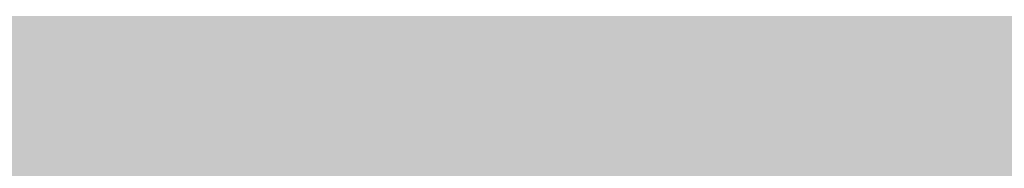
# Model space of a CAD drawing. Units: feet. Extents: x 3168 to 4724, y 827 to 1477.
# Tile 175 of 256: x 3303.032 to 3307.378, y 1098.344 to 1099.001. Entities that reach past the tile are written whole.
import ezdxf

# ---------------------------------------------------------------- set-up
doc = ezdxf.new("R2010")
doc.units = ezdxf.units.FT
doc.layers.add('A-ELEV', color=7, linetype='Continuous', lineweight=35)
doc.layers.add('A-ELEV-PATT', color=8, linetype='Continuous', lineweight=13)

msp = doc.modelspace()

# ---------------------------------------------------------------- hatches: boundary and pattern name
at = {"layer": 'A-ELEV-PATT'}
h = msp.add_hatch(color=256, dxfattribs=at)
h.dxf.hatch_style = 1
edge = h.paths.add_edge_path()
edge.add_ellipse((3552.9058, 979.2201), major_axis=(36.7449, 0), ratio=0.4848485, start_angle=0, end_angle=360)
edge = h.paths.add_edge_path()
edge.add_ellipse((3559.8916, 929.2523), major_axis=(36.7449, 0), ratio=0.4848485, start_angle=0, end_angle=360)
edge = h.paths.add_edge_path()
edge.add_line((3299.3168, 1198.6061), (3479.9167, 1198.6061))
edge.add_line((3479.9167, 1198.6061), (3479.9167, 1209.8686))
edge.add_spline(control_points=[(3479.9167, 1209.8686), (3464.3012, 1209.8686), (3448.6856, 1209.8686), (3410.9491, 1209.8686), (3388.8282, 1209.8686), (3355.6469, 1209.8686), (3344.5864, 1209.8686), (3327.9957, 1209.8686), (3322.4655, 1209.8686), (3314.1702, 1209.8686), (3311.4051, 1209.8686), (3307.2574, 1209.8686), (3305.8748, 1209.8686), (3303.801, 1209.8686), (3303.1097, 1209.8686), (3302.0728, 1209.8686), (3301.7272, 1209.8686), (3301.2087, 1209.8686), (3301.0359, 1209.8686), (3300.7767, 1209.8686), (3300.6903, 1209.8686), (3300.5606, 1209.8686), (3300.5174, 1209.8686), (3300.4526, 1209.8686), (3300.431, 1209.8686), (3300.3986, 1209.8686), (3300.3878, 1209.8686), (3300.3662, 1209.8686), (3300.3457, 1209.8686), (3300.3455, 1209.8686), (3300.3455, 1209.8686), (3300.3433, 1209.8686), (3300.3411, 1209.8686), (3300.3379, 1209.8686), (3300.3368, 1209.8686), (3300.3339, 1209.8686), (3300.3321, 1209.8686), (3300.3255, 1209.8686), (3300.3207, 1209.8686), (3300.3109, 1209.8686), (3300.306, 1209.8686), (3300.2905, 1209.8686), (3300.28, 1209.8686), (3300.2324, 1209.8688), (3300.1953, 1209.869), (3299.9511, 1209.8706), (3299.7448, 1209.8743), (3299.4368, 1209.8833), (3299.3344, 1209.8868), (3299.1811, 1209.8929), (3299.13, 1209.8951), (3298.6522, 1209.9168), (3298.2295, 1209.9457), (3297.6016, 1210.0024), (3297.3934, 1210.0235), (3297.0827, 1210.0583), (3296.9793, 1210.0705), (3296.293, 1210.1549), (3295.7181, 1210.2434), (3294.8687, 1210.3989), (3294.5877, 1210.4545), (3294.1693, 1210.5433), (3294.0304, 1210.5739), (3291.7071, 1211.1012), (3289.6536, 1211.8134), (3285.7763, 1213.564), (3283.9514, 1214.6035), (3280.5122, 1216.9801), (3278.8972, 1218.3176), (3276.3799, 1220.8295), (3275.416, 1221.9177), (3274.0393, 1223.7077), (3273.581, 1224.3495), (3273.1432, 1225.0163)], knot_values=[39.119033, 39.119033, 39.119033, 39.119033, 39.286353, 39.286353, 39.523379, 39.523379, 39.641892, 39.641892, 39.701148, 39.701148, 39.730777, 39.730777, 39.745591, 39.745591, 39.752998, 39.752998, 39.756701, 39.756701, 39.758553, 39.758553, 39.759479, 39.759479, 39.759942, 39.759942, 39.760173, 39.760173, 39.760289, 39.760289, 39.760405, 39.760405, 39.760463, 39.760463, 39.763389, 39.763389, 39.764851, 39.764851, 39.767304, 39.767304, 39.773825, 39.773825, 39.78057, 39.78057, 39.79477, 39.79477, 39.845194, 39.845194, 40.126715, 40.126715, 40.267476, 40.267476, 40.337856, 40.337856, 40.927023, 40.927023, 41.221606, 41.221606, 41.368898, 41.368898, 42.202622, 42.202622, 42.619485, 42.619485, 42.827916, 42.827916, 46.118323, 46.118323, 49.408731, 49.408731, 52.699139, 52.699139, 54.927489, 54.927489, 56.104228, 56.104228, 56.104228, 56.104228], weights=[1, 1, 1, 1, 1, 1, 1, 1, 1, 1, 1, 1, 1, 1, 1, 1, 1, 1, 1, 1, 1, 1, 1, 1, 1, 1, 1, 1, 1, 1, 1, 1, 1, 1, 1, 1, 1, 1, 1, 1, 1, 1, 1, 1, 1, 1, 1, 1, 1, 1, 1, 1, 1, 1, 1, 1, 1, 1, 1, 1, 1, 1, 1, 1, 1, 1, 1, 1, 1, 1, 1, 1, 1, 1], degree=3, periodic=0)
edge.add_line((3273.1432, 1225.0163), (3273.1432, 1099.0163))
edge.add_line((3273.1432, 1099.0163), (3299.3168, 1099.0163))
edge.add_line((3299.3168, 1099.0163), (3299.3168, 1198.6061))
edge = h.paths.add_edge_path()
edge.add_line((3304.7584, 1324.1581), (3479.9167, 1324.1581))
edge.add_line((3479.9167, 1324.1581), (3479.9167, 1335.7146))
edge.add_line((3479.9167, 1335.7146), (3269.1616, 1335.7146))
edge.add_spline(control_points=[(3269.1616, 1335.7146), (3264.0242, 1335.7146), (3258.3641, 1328.9582), (3259.2643, 1323.9003)], knot_values=[0, 0, 0, 0, 15.412191, 15.412191, 15.412191, 15.412191], degree=3, periodic=0)
edge.add_line((3259.2643, 1323.9003), (3265.5168, 1288.7691))
edge.add_line((3265.5168, 1288.7691), (3275.2651, 1261.5456))
edge.add_line((3275.2651, 1261.5456), (3304.7584, 1261.5456))
edge.add_line((3304.7584, 1261.5456), (3304.7584, 1324.1581))
h = msp.add_hatch(color=256, dxfattribs=at)
h.dxf.hatch_style = 1
h.paths.add_polyline_path([(3384.5252, 1099.0163), (3335.0292, 1099.0163), (3299.3168, 1099.0163), (3273.1432, 1099.0163), (3217.5654, 1099.0163), (3168.0693, 827.1163), (3335.0292, 827.1163)])

# ---------------------------------------------------------------- linework, layer by layer
at = {"layer": 'A-ELEV'}
msp.add_open_spline([(3808.5202, 1099.0163), (3808.5202, 1141.4132), (3808.5202, 1183.8102), (3808.5202, 1226.6353), (3808.5202, 1227.0636), (3808.5202, 1227.4918), (3811.4919, 1248.9947), (3814.4635, 1270.4975), (3817.4652, 1292.2176), (3817.4952, 1292.4348), (3817.5253, 1292.652), (3817.5728, 1310.1067), (3817.6203, 1327.5615), (3817.6679, 1345.0163), (3817.6679, 1345.458), (3817.6679, 1345.8996), (3817.6679, 1346.456), (3817.6679, 1346.5708), (3817.6679, 1346.7529), (3817.6679, 1346.8201), (3817.6679, 1346.9349), (3817.6679, 1346.9823), (3817.6679, 1347.0386), (3817.6679, 1347.0474), (3817.6679, 1347.0737), (3817.6679, 1347.0593), (3817.6679, 1347.0615), (3817.6679, 1347.0627), (3817.6679, 1347.066), (3817.6679, 1347.0683), (3817.6679, 1347.075), (3817.6679, 1347.0795), (3817.6678, 1347.0929), (3817.6678, 1347.1019), (3817.6678, 1347.1288), (3817.6677, 1347.1467), (3817.6674, 1347.2004), (3817.6672, 1347.2362), (3817.6661, 1347.3434), (3817.665, 1347.4147), (3817.6608, 1347.6281), (3817.6566, 1347.7697), (3817.64, 1348.1925), (3817.6235, 1348.4716), (3817.5591, 1349.3001), (3817.4961, 1349.8406), (3817.2554, 1351.4242), (3817.0263, 1352.4288), (3816.3069, 1354.8889), (3815.7437, 1356.2687), (3814.464, 1358.8192), (3813.7464, 1359.991), (3812.1958, 1362.1723), (3811.3622, 1363.1821), (3809.5888, 1365.069), (3808.6488, 1365.9461), (3806.6543, 1367.5796), (3805.5997, 1368.3362), (3803.3529, 1369.7223), (3802.1605, 1370.3524), (3799.6008, 1371.4536), (3798.2327, 1371.9255), (3795.2801, 1372.6346), (3793.6931, 1372.8721), (3791.8694, 1372.9265), (3791.7409, 1372.9292), (3791.3534, 1372.9341), (3791.0927, 1372.9329), (3790.3041, 1372.9151), (3789.7695, 1372.8842), (3789.2092, 1372.8302), (3789.1906, 1372.8284), (3789.1349, 1372.8229), (3789.0977, 1372.8191), (3789.0484, 1372.814), (3789.0364, 1372.8127), (3789.0003, 1372.8089), (3788.9761, 1372.8063), (3788.9494, 1372.8034), (3788.9468, 1372.8031), (3788.9426, 1372.8027), (3788.941, 1372.8025), (3788.9386, 1372.8022), (3788.9378, 1372.8021), (3788.9354, 1372.8019), (3788.8675, 1372.7944), (3788.7569, 1372.7822), (3788.7015, 1372.7761), (3788.5355, 1372.7579), (3788.4249, 1372.7457), (3788.0929, 1372.7092), (3787.8715, 1372.6848), (3787.2075, 1372.6118), (3786.7648, 1372.5631), (3785.4368, 1372.417), (3784.5515, 1372.3196), (3781.8954, 1372.0274), (3780.1247, 1371.8327), (3774.8126, 1371.2483), (3771.2713, 1370.8587), (3760.6471, 1369.69), (3753.5643, 1368.9109), (3732.316, 1366.5735), (3718.1504, 1365.0152), (3694.0068, 1362.3593), (3684.0287, 1361.2617), (3674.0506, 1360.1641), (3664.6007, 1360.1641), (3655.1508, 1360.1641), (3626.8011, 1360.1641), (3607.9013, 1360.1641), (3551.2019, 1360.1641), (3513.4023, 1360.1641), (3467.7252, 1360.1641), (3459.8476, 1360.1641), (3436.2149, 1360.1641), (3420.4597, 1360.1641), (3373.1943, 1360.1641), (3341.6839, 1360.1641), (3302.8482, 1360.1641), (3295.5227, 1360.1641), (3286.0383, 1360.1641), (3283.8794, 1360.1641), (3277.4026, 1360.1641), (3273.0848, 1360.1641), (3267.7329, 1360.1641), (3266.6988, 1360.1641), (3263.5965, 1360.1641), (3261.5284, 1360.1641), (3259.2369, 1360.1641), (3259.0137, 1360.1641), (3258.344, 1360.1641), (3257.8975, 1360.1641), (3257.431, 1360.1641), (3257.411, 1360.1641), (3257.3706, 1360.1641), (3257.3755, 1360.1641), (3257.3746, 1360.1641), (3257.3739, 1360.1641), (3257.372, 1360.1641), (3257.3706, 1360.1641), (3257.3667, 1360.1641), (3257.364, 1360.1641), (3257.3561, 1360.1641), (3257.3508, 1360.164), (3257.335, 1360.164), (3257.3244, 1360.164), (3257.2928, 1360.1639), (3257.2717, 1360.1638), (3257.2084, 1360.1634), (3257.1663, 1360.163), (3257.0402, 1360.1614), (3256.9563, 1360.1598), (3256.7055, 1360.1534), (3256.5392, 1360.147), (3256.0436, 1360.1219), (3255.7173, 1360.0971), (3254.7524, 1360.0005), (3254.128, 1359.9065), (3252.1801, 1359.5253), (3250.9416, 1359.144), (3248.6702, 1358.2433), (3247.6357, 1357.7238), (3245.7326, 1356.6035), (3244.8634, 1356.0021), (3243.2531, 1354.7429), (3242.512, 1354.0847), (3240.7511, 1352.3448), (3239.801, 1351.2296), (3238.0878, 1348.8724), (3237.3247, 1347.6304), (3235.9825, 1344.9716), (3235.4022, 1343.5549), (3234.5911, 1340.8155), (3234.3109, 1339.5435), (3233.9765, 1336.8026), (3233.9221, 1335.3309), (3234.1489, 1332.5913), (3234.3495, 1331.3672), (3234.7199, 1329.9994), (3234.7524, 1329.8834), (3234.8536, 1329.5348), (3234.9259, 1329.3017), (3235.0248, 1329.0026), (3235.0469, 1328.9369), (3235.0776, 1328.8472), (3235.0859, 1328.8232), (3235.1109, 1328.7511), (3235.1278, 1328.703), (3235.148, 1328.6462), (3235.1511, 1328.6376), (3235.1561, 1328.6235), (3235.1581, 1328.618), (3235.1602, 1328.612), (3235.1656, 1328.5969), (3235.1801, 1328.5565), (3235.1903, 1328.5281), (3235.2208, 1328.4429), (3235.2411, 1328.3862), (3235.3021, 1328.2159), (3235.3427, 1328.1023), (3235.4647, 1327.7617), (3235.546, 1327.5346), (3235.79, 1326.8534), (3235.9526, 1326.3992), (3236.4405, 1325.0367), (3236.7657, 1324.1284), (3237.7415, 1321.4034), (3238.392, 1319.5868), (3240.3435, 1314.1369), (3241.6445, 1310.5036), (3245.5476, 1299.6037), (3248.1496, 1292.3371), (3255.9557, 1270.5374), (3261.1598, 1256.0042), (3267.3876, 1238.612), (3268.4114, 1235.7529), (3269.5104, 1232.6839), (3269.5856, 1232.4739), (3269.7066, 1232.1359), (3269.7524, 1232.0079), (3269.8273, 1231.7987), (3269.8564, 1231.7176), (3269.9063, 1231.5781), (3269.9272, 1231.5198), (3269.9725, 1231.3934), (3269.9968, 1231.3254), (3270.0265, 1231.2425), (3270.0318, 1231.2277), (3270.0403, 1231.204), (3270.0392, 1231.207), (3270.0394, 1231.2066), (3270.0394, 1231.2064), (3270.0396, 1231.2058), (3270.0398, 1231.2055), (3270.0402, 1231.2043), (3270.0404, 1231.2036), (3270.0413, 1231.2013), (3270.0418, 1231.1998), (3270.0434, 1231.1953), (3270.0445, 1231.1922), (3270.0478, 1231.1832), (3270.0499, 1231.1771), (3270.0564, 1231.159), (3270.0608, 1231.147), (3270.0739, 1231.1108), (3270.0826, 1231.0867), (3270.1089, 1231.0144), (3270.1266, 1230.9663), (3270.1799, 1230.8225), (3270.2159, 1230.7269), (3270.3253, 1230.4415), (3270.4, 1230.2528), (3270.6292, 1229.6914), (3270.7889, 1229.3235), (3271.2865, 1228.2383), (3271.6431, 1227.5398), (3272.7759, 1225.5153), (3273.6142, 1224.2605), (3275.416, 1221.9177), (3276.3799, 1220.8295), (3278.8972, 1218.3176), (3280.5122, 1216.9801), (3283.9514, 1214.6035), (3285.7763, 1213.564), (3289.6536, 1211.8134), (3291.7071, 1211.1012), (3294.0304, 1210.5739), (3294.1693, 1210.5433), (3294.5877, 1210.4545), (3294.8687, 1210.3989), (3295.7181, 1210.2434), (3296.293, 1210.1549), (3296.9793, 1210.0705), (3297.0827, 1210.0583), (3297.3934, 1210.0235), (3297.6016, 1210.0024), (3298.2295, 1209.9457), (3298.6522, 1209.9168), (3299.13, 1209.8951), (3299.1811, 1209.8929), (3299.3344, 1209.8868), (3299.4368, 1209.8833), (3299.7448, 1209.8743), (3299.9511, 1209.8706), (3300.1953, 1209.869), (3300.2324, 1209.8688), (3300.28, 1209.8686), (3300.2905, 1209.8686), (3300.306, 1209.8686), (3300.3109, 1209.8686), (3300.3207, 1209.8686), (3300.3255, 1209.8686), (3300.3321, 1209.8686), (3300.3339, 1209.8686), (3300.3368, 1209.8686), (3300.3379, 1209.8686), (3300.3411, 1209.8686), (3300.3433, 1209.8686), (3300.3455, 1209.8686), (3300.3455, 1209.8686), (3300.3457, 1209.8686), (3300.3662, 1209.8686), (3300.3878, 1209.8686), (3300.3986, 1209.8686), (3300.431, 1209.8686), (3300.4526, 1209.8686), (3300.5174, 1209.8686), (3300.5606, 1209.8686), (3300.6903, 1209.8686), (3300.7767, 1209.8686), (3301.0359, 1209.8686), (3301.2087, 1209.8686), (3301.7272, 1209.8686), (3302.0728, 1209.8686), (3303.1097, 1209.8686), (3303.801, 1209.8686), (3305.8748, 1209.8686), (3307.2574, 1209.8686), (3311.4051, 1209.8686), (3314.1702, 1209.8686), (3322.4655, 1209.8686), (3327.9957, 1209.8686), (3344.5864, 1209.8686), (3355.6469, 1209.8686), (3388.8282, 1209.8686), (3410.9491, 1209.8686), (3477.3119, 1209.8686), (3521.5537, 1209.8686), (3566.8362, 1209.8686), (3567.8769, 1209.8686), (3570.999, 1209.8686), (3573.0804, 1209.8686), (3575.7814, 1209.8686), (3576.4009, 1209.8686), (3577.2958, 1209.8686), (3577.5712, 1209.8686), (3578.3971, 1209.8686), (3578.9478, 1209.8686), (3579.7565, 1209.8686), (3580.0145, 1209.8686), (3580.3427, 1209.8686), (3580.3269, 1209.8686), (3580.3272, 1209.8686), (3580.3273, 1209.8686), (3580.3278, 1209.8686), (3580.3281, 1209.8686), (3580.329, 1209.8686), (3580.3296, 1209.8686), (3580.3314, 1209.8686), (3580.3327, 1209.8686), (3580.3363, 1209.8686), (3580.3388, 1209.8686), (3580.3461, 1209.8686), (3580.351, 1209.8686), (3580.3657, 1209.8685), (3580.3754, 1209.8685), (3580.4048, 1209.8684), (3580.4244, 1209.8684), (3580.4832, 1209.8681), (3580.5224, 1209.8678), (3580.6404, 1209.8666), (3580.7192, 1209.8655), (3580.9563, 1209.8608), (3581.1152, 1209.8561), (3581.5942, 1209.8372), (3581.9164, 1209.8183), (3582.8899, 1209.7424), (3583.548, 1209.6662), (3585.5318, 1209.3606), (3586.8672, 1209.0539), (3589.4715, 1208.2525), (3590.7402, 1207.7579), (3591.9955, 1207.1588), (3592.0578, 1207.1287), (3592.2442, 1207.038), (3592.3677, 1206.9766), (3592.7353, 1206.7904), (3592.9768, 1206.6631), (3593.2445, 1206.5164), (3593.2747, 1206.4998), (3593.3651, 1206.4498), (3593.4251, 1206.4163), (3593.6043, 1206.3153), (3593.7227, 1206.2472), (3593.8572, 1206.1684), (3593.8744, 1206.1583), (3593.9257, 1206.128), (3593.9599, 1206.1078), (3594.0621, 1206.0469), (3594.1298, 1206.0061), (3594.2084, 1205.9582), (3594.2197, 1205.9513), (3594.2534, 1205.9307), (3594.2758, 1205.9169), (3594.343, 1205.8755), (3594.3876, 1205.8479), (3594.4336, 1205.819), (3594.4353, 1205.818), (3594.4402, 1205.8149), (3594.4435, 1205.8129), (3594.4471, 1205.8106), (3594.4475, 1205.8103), (3594.4487, 1205.8096), (3594.4495, 1205.8091), (3594.4504, 1205.8086), (3594.4505, 1205.8085), (3594.4506, 1205.8084), (3594.4674, 1205.7979), (3594.4933, 1205.7817), (3594.5062, 1205.7736), (3594.545, 1205.7492), (3594.5709, 1205.733), (3594.6485, 1205.6844), (3594.7002, 1205.652), (3594.8554, 1205.5547), (3594.9589, 1205.4898), (3595.2694, 1205.2953), (3595.4763, 1205.1656), (3596.0972, 1204.7765), (3596.5111, 1204.5171), (3597.7528, 1203.7388), (3598.5807, 1203.22), (3601.0642, 1201.6636), (3602.7198, 1200.6259), (3607.6868, 1197.513), (3610.9981, 1195.4377), (3620.932, 1189.2119), (3627.5546, 1185.0614), (3647.4225, 1172.6097), (3660.6678, 1164.3086), (3700.4035, 1139.4053), (3726.894, 1122.8031), (3757.2057, 1103.8061), (3761.027, 1101.4112), (3764.8482, 1099.0163), (3745.3283, 1099.0163), (3725.8083, 1099.0163), (3706.2884, 1099.0163), (3706.2884, 1108.4532), (3706.2884, 1117.8902), (3706.2884, 1127.3271), (3710.7508, 1127.3271), (3715.2131, 1127.3271), (3719.6755, 1127.3271)], degree=3, knots=[0, 0, 0, 0, 0.982037, 0.982037, 0.991957, 0.991957, 0.991957, 1.966522, 1.966522, 1.976367, 1.976367, 1.976367, 2.976367, 2.976367, 2.976367, 3.00169, 3.00169, 3.008272, 3.008272, 3.012129, 3.012129, 3.014851, 3.014851, 3.015353, 3.015353, 3.016359, 3.016359, 3.017365, 3.017365, 3.019376, 3.019376, 3.023398, 3.023398, 3.031442, 3.031442, 3.047531, 3.047531, 3.079708, 3.079708, 3.144063, 3.144063, 3.272772, 3.272772, 3.53019, 3.53019, 4.045026, 4.045026, 5.074698, 5.074698, 6.700878, 6.700878, 8.327058, 8.327058, 9.953238, 9.953238, 11.579418, 11.579418, 13.205598, 13.205598, 14.831778, 14.831778, 16.457958, 16.457958, 18.084138, 18.084138, 18.206872, 18.206872, 18.45234, 18.45234, 18.943275, 18.943275, 18.960093, 18.960093, 18.993729, 18.993729, 19.00461, 19.00461, 19.026374, 19.026374, 19.028737, 19.028737, 19.03018, 19.03018, 19.030897, 19.030897, 19.032332, 19.032332, 19.033766, 19.033766, 19.036636, 19.036636, 19.042374, 19.042374, 19.053851, 19.053851, 19.076805, 19.076805, 19.122714, 19.122714, 19.21453, 19.21453, 19.398163, 19.398163, 19.765429, 19.765429, 20.024128, 20.024128, 20.024128, 20.092031, 20.092031, 20.227836, 20.227836, 20.499446, 20.499446, 20.556051, 20.556051, 20.66926, 20.66926, 20.895678, 20.895678, 20.948316, 20.948316, 20.963829, 20.963829, 20.994855, 20.994855, 21.002285, 21.002285, 21.017146, 21.017146, 21.01875, 21.01875, 21.021959, 21.021959, 21.022102, 21.022102, 21.022249, 21.022249, 21.022708, 21.022708, 21.023627, 21.023627, 21.025464, 21.025464, 21.029138, 21.029138, 21.036486, 21.036486, 21.051183, 21.051183, 21.080575, 21.080575, 21.139361, 21.139361, 21.256932, 21.256932, 21.492073, 21.492073, 21.962356, 21.962356, 23.01002, 23.01002, 24.057684, 24.057684, 25.105348, 25.105348, 26.153011, 26.153011, 27.776787, 27.776787, 29.400562, 29.400562, 31.024337, 31.024337, 32.278801, 32.278801, 33.533265, 33.533265, 34.467568, 34.467568, 34.553971, 34.553971, 34.726776, 34.726776, 34.775309, 34.775309, 34.793079, 34.793079, 34.82862, 34.82862, 34.834979, 34.834979, 34.839039, 34.839039, 34.839411, 34.839411, 34.840285, 34.840285, 34.842034, 34.842034, 34.845531, 34.845531, 34.852525, 34.852525, 34.866512, 34.866512, 34.894488, 34.894488, 34.950439, 34.950439, 35.062342, 35.062342, 35.286147, 35.286147, 35.733758, 35.733758, 35.821815, 35.821815, 35.828283, 35.828283, 35.832225, 35.832225, 35.834724, 35.834724, 35.836521, 35.836521, 35.838617, 35.838617, 35.839073, 35.839073, 35.839345, 35.839345, 35.839617, 35.839617, 35.840161, 35.840161, 35.841249, 35.841249, 35.843425, 35.843425, 35.847778, 35.847778, 35.856482, 35.856482, 35.873891, 35.873891, 35.908709, 35.908709, 35.978345, 35.978345, 36.117617, 36.117617, 36.396161, 36.396161, 36.953248, 36.953248, 38.067423, 38.067423, 40.295772, 40.295772, 42.524122, 42.524122, 45.81453, 45.81453, 49.104937, 49.104937, 52.395345, 52.395345, 52.603776, 52.603776, 53.020639, 53.020639, 53.854363, 53.854363, 54.001655, 54.001655, 54.296238, 54.296238, 54.885405, 54.885405, 54.955785, 54.955785, 55.096546, 55.096546, 55.378067, 55.378067, 55.42849, 55.42849, 55.442691, 55.442691, 55.449436, 55.449436, 55.455957, 55.455957, 55.458409, 55.458409, 55.459872, 55.459872, 55.462798, 55.462798, 55.462856, 55.462856, 55.462972, 55.462972, 55.463088, 55.463088, 55.463319, 55.463319, 55.463782, 55.463782, 55.464708, 55.464708, 55.46656, 55.46656, 55.470263, 55.470263, 55.47767, 55.47767, 55.492484, 55.492484, 55.522112, 55.522112, 55.581369, 55.581369, 55.699882, 55.699882, 55.936907, 55.936907, 56.410959, 56.410959, 56.42211, 56.42211, 56.444413, 56.444413, 56.451051, 56.451051, 56.454001, 56.454001, 56.459901, 56.459901, 56.462666, 56.462666, 56.463418, 56.463418, 56.464171, 56.464171, 56.465675, 56.465675, 56.468684, 56.468684, 56.474702, 56.474702, 56.486738, 56.486738, 56.51081, 56.51081, 56.558955, 56.558955, 56.655243, 56.655243, 56.847821, 56.847821, 57.232975, 57.232975, 58.003284, 58.003284, 59.543901, 59.543901, 62.625137, 62.625137, 68.787607, 68.787607, 74.950078, 74.950078, 75.27336, 75.27336, 75.919923, 75.919923, 77.213051, 77.213051, 77.377769, 77.377769, 77.707206, 77.707206, 78.366079, 78.366079, 78.462532, 78.462532, 78.655436, 78.655436, 79.041245, 79.041245, 79.105735, 79.105735, 79.234714, 79.234714, 79.492672, 79.492672, 79.502197, 79.502197, 79.521249, 79.521249, 79.523534, 79.523534, 79.528103, 79.528103, 79.528682, 79.528682, 79.528885, 79.528885, 79.529089, 79.529089, 79.529495, 79.529495, 79.530308, 79.530308, 79.531935, 79.531935, 79.535187, 79.535187, 79.541693, 79.541693, 79.554704, 79.554704, 79.580725, 79.580725, 79.632769, 79.632769, 79.736856, 79.736856, 79.94503, 79.94503, 80.361377, 80.361377, 80.421435, 80.421435, 80.421435, 81.421435, 81.421435, 81.421435, 82.421435, 82.421435, 82.421435, 83.421435, 83.421435, 83.421435, 83.421435], dxfattribs=at)

doc.saveas('drawing.dxf')
